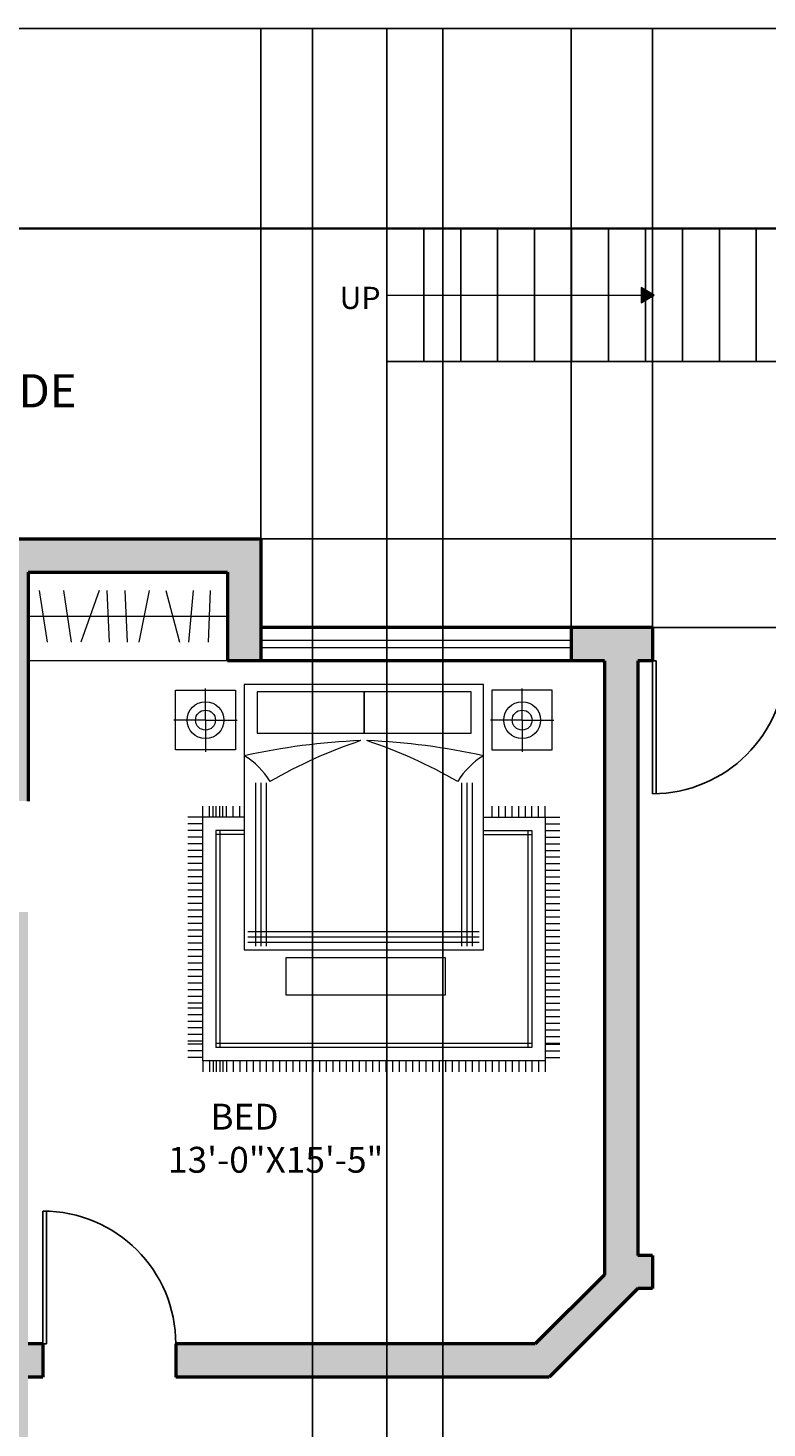
# Model space of a CAD drawing. Units: inches. Extents: x 2447 to 3157, y 2799 to 3988.
# Tile 8 of 9: x 2735 to 2935, y 3609 to 3988. Entities that reach past the tile are written whole.
import ezdxf

# ---------------------------------------------------------------- set-up
doc = ezdxf.new("R2010")
doc.units = ezdxf.units.IN
for name, color, linetype, lineweight in [('A-ANNO-DIMS', 2, 'Continuous', 18), ('A-ANNO-SYMB', 2, 'Continuous', 18), ('A-AREA-IDEN', 7, 'Continuous', 25), ('A-DOOR', 3, 'Continuous', 25), ('A-FLOR-CASE', 8, 'Continuous', 20), ('A-FLOR-STRS', 7, 'Continuous', 25), ('A-FURN', 8, 'Continuous', 18), ('A-GLAZ', 4, 'Continuous', 18), ('A-WALL', 7, 'Continuous', 50), ('A-WALL-PATT', 252, 'Continuous', 13), ('C-PROP', 6, 'Continuous', 35)]:
    doc.layers.add(name, color=color, linetype=linetype, lineweight=lineweight)
doc.styles.get("Standard").update_dxf_attribs({"font": 'arial.ttf'})
doc.dimstyles.get("Standard").update_dxf_attribs({"dimtxt": 0.18, "dimasz": 0.18, "dimexe": 0.18, "dimexo": 0.0625, "dimgap": 0.09, "dimtad": 0, "dimtih": 1, "dimtoh": 1, "dimdec": 4, "dimzin": 0, "dimdsep": 46, "dimtxsty": 'Standard', "dimcen": 0.09, "dimadec": 0, "dimazin": 0, "dimtfac": 1, "dimtdec": 4, "dimtofl": 0, "dimtmove": 0, "dimatfit": 3, "dimfxl": 1, "dimtolj": 1, "dimtzin": 0, "dimarcsym": 0})

# ---------------------------------------------------------------- blocks, each defined once
blk = doc.blocks.new('A$C462B680F')
for p, q in [((0.011, 2.874, -0.291), (0.465, 2.874, -0.291)), ((0.011, 2.424, -0.291), (0.011, 2.874, -0.291)), ((0.238, 2.649, -0.561), (0.238, 2.887, -0.561)), ((0.465, 2.874, -0.291), (0.465, 2.424, -0.291)), ((2.33, 2.918, -0.291), (0.53, 2.918, -0.291)), ((0.53, 2.918, -0.291), (0.53, 0.918, -0.291)), ((1.434, 2.861, -0.291), (0.627, 2.861, -0.291)), ((0.627, 2.861, -0.291), (0.627, 2.55, -0.291)), ((1.43, 2.861, -0.291), (1.43, 2.55, -0.291)), ((2.237, 2.861, -0.291), (1.43, 2.861, -0.291)), ((1.434, 2.55, -0.291), (1.434, 2.861, -0.291)), ((2.237, 2.55, -0.291), (2.237, 2.861, -0.291)), ((2.33, 0.918, -0.291), (2.33, 2.918, -0.291)), ((2.849, 2.874, -0.291), (2.395, 2.874, -0.291)), ((2.395, 2.874, -0.291), (2.395, 2.424, -0.291)), ((2.622, 2.649, -0.561), (2.622, 2.887, -0.561)), ((2.849, 2.424, -0.291), (2.849, 2.874, -0.291)), ((0.238, 2.649, -0.561), (0, 2.649, -0.561)), ((0.238, 2.649, -0.561), (0.238, 2.411, -0.561)), ((0.238, 2.649, -0.561), (0.476, 2.649, -0.561)), ((2.622, 2.649, -0.561), (2.384, 2.649, -0.561)), ((2.622, 2.649, -0.561), (2.622, 2.411, -0.561)), ((2.622, 2.649, -0.561), (2.861, 2.649, -0.561)), ((0.627, 2.55, -0.291), (1.434, 2.55, -0.291)), ((1.43, 2.55, -0.291), (2.237, 2.55, -0.291)), ((0.465, 2.424, -0.291), (0.011, 2.424, -0.291)), ((2.395, 2.424, -0.291), (2.849, 2.424, -0.291)), ((0.615, 2.176, -0.291), (0.615, 0.947, -0.291)), ((0.655, 2.176, -0.291), (0.655, 0.947, -0.291)), ((0.695, 2.176, -0.291), (0.695, 0.947, -0.291)), ((2.165, 2.176, -0.291), (2.165, 0.947, -0.291)), ((2.205, 2.176, -0.291), (2.205, 0.947, -0.291)), ((2.245, 2.176, -0.291), (2.245, 0.947, -0.291)), ((0.215, 1.918, -0.291), (0.105, 1.918, -0.291)), ((0.215, 1.918, -0.291), (0.215, 0.082, -0.291)), ((0.53, 1.918, -0.291), (0.215, 1.918, -0.291)), ((0.219, 1.918, -0.291), (0.219, 2, -0.291)), ((0.269, 1.918, -0.291), (0.269, 2, -0.291)), ((0.296, 1.918, -0.291), (0.296, 2, -0.291)), ((0.319, 1.918, -0.291), (0.319, 2, -0.291)), ((0.346, 1.918, -0.291), (0.346, 2, -0.291)), ((0.369, 1.918, -0.291), (0.369, 2, -0.291)), ((0.396, 1.918, -0.291), (0.396, 2, -0.291)), ((0.446, 1.918, -0.291), (0.446, 2, -0.291)), ((0.496, 1.918, -0.291), (0.496, 2, -0.291)), ((2.33, 1.918, -0.291), (2.796, 1.918, -0.291)), ((2.396, 1.918, -0.291), (2.396, 2, -0.291)), ((2.446, 1.918, -0.291), (2.446, 2, -0.291)), ((2.496, 1.918, -0.291), (2.496, 2, -0.291)), ((2.546, 1.918, -0.291), (2.546, 2, -0.291)), ((2.596, 1.918, -0.291), (2.596, 2, -0.291)), ((2.646, 1.918, -0.291), (2.646, 2, -0.291)), ((2.696, 1.918, -0.291), (2.696, 2, -0.291)), ((2.746, 1.918, -0.291), (2.746, 2, -0.291)), ((2.796, 1.918, -0.291), (2.796, 2, -0.291)), ((2.796, 1.918, -0.291), (2.796, 0.082, -0.291)), ((2.796, 1.918, -0.291), (2.906, 1.918, -0.291)), ((0.215, 1.868, -0.291), (0.105, 1.868, -0.291)), ((0.215, 1.818, -0.291), (0.105, 1.818, -0.291)), ((0.315, 1.818, -0.291), (0.315, 0.182, -0.291)), ((0.53, 1.818, -0.291), (0.315, 1.818, -0.291)), ((0.345, 1.818, -0.291), (0.345, 0.182, -0.291)), ((2.33, 1.818, -0.291), (2.696, 1.818, -0.291)), ((2.666, 1.818, -0.291), (2.666, 0.182, -0.291)), ((2.696, 1.818, -0.291), (2.696, 0.182, -0.291)), ((2.796, 1.868, -0.291), (2.906, 1.868, -0.291)), ((2.796, 1.818, -0.291), (2.906, 1.818, -0.291)), ((0.215, 1.768, -0.291), (0.105, 1.768, -0.291)), ((0.215, 1.718, -0.291), (0.105, 1.718, -0.291)), ((0.53, 1.788, -0.291), (0.315, 1.788, -0.291)), ((2.33, 1.788, -0.291), (2.696, 1.788, -0.291)), ((2.796, 1.768, -0.291), (2.906, 1.768, -0.291)), ((2.796, 1.718, -0.291), (2.906, 1.718, -0.291)), ((0.215, 1.668, -0.291), (0.105, 1.668, -0.291)), ((0.215, 1.618, -0.291), (0.105, 1.618, -0.291)), ((2.796, 1.668, -0.291), (2.906, 1.668, -0.291)), ((2.796, 1.618, -0.291), (2.906, 1.618, -0.291)), ((0.215, 1.568, -0.291), (0.105, 1.568, -0.291)), ((0.215, 1.518, -0.291), (0.105, 1.518, -0.291)), ((2.796, 1.568, -0.291), (2.906, 1.568, -0.291)), ((2.796, 1.518, -0.291), (2.906, 1.518, -0.291)), ((0.215, 1.468, -0.291), (0.105, 1.468, -0.291)), ((0.215, 1.418, -0.291), (0.105, 1.418, -0.291)), ((2.796, 1.468, -0.291), (2.906, 1.468, -0.291)), ((2.796, 1.418, -0.291), (2.906, 1.418, -0.291)), ((0.215, 1.368, -0.291), (0.105, 1.368, -0.291)), ((0.215, 1.318, -0.291), (0.105, 1.318, -0.291)), ((0.215, 1.268, -0.291), (0.105, 1.268, -0.291)), ((2.796, 1.368, -0.291), (2.906, 1.368, -0.291)), ((2.796, 1.318, -0.291), (2.906, 1.318, -0.291)), ((2.796, 1.268, -0.291), (2.906, 1.268, -0.291)), ((0.215, 1.218, -0.291), (0.105, 1.218, -0.291)), ((0.215, 1.168, -0.291), (0.105, 1.168, -0.291)), ((2.796, 1.218, -0.291), (2.906, 1.218, -0.291)), ((2.796, 1.168, -0.291), (2.906, 1.168, -0.291)), ((0.215, 1.118, -0.291), (0.105, 1.118, -0.291)), ((0.215, 1.068, -0.291), (0.105, 1.068, -0.291)), ((0.558, 1.057, -0.291), (2.299, 1.057, -0.291)), ((2.796, 1.118, -0.291), (2.906, 1.118, -0.291)), ((2.796, 1.068, -0.291), (2.906, 1.068, -0.291)), ((0.215, 1.018, -0.291), (0.105, 1.018, -0.291)), ((0.215, 0.968, -0.291), (0.105, 0.968, -0.291)), ((0.558, 1.017, -0.291), (2.299, 1.017, -0.291)), ((0.558, 0.977, -0.291), (2.299, 0.977, -0.291)), ((2.796, 1.018, -0.291), (2.906, 1.018, -0.291)), ((2.796, 0.968, -0.291), (2.906, 0.968, -0.291)), ((0.215, 0.918, -0.291), (0.105, 0.918, -0.291)), ((0.215, 0.868, -0.291), (0.105, 0.868, -0.291)), ((0.53, 0.918, -0.291), (2.33, 0.918, -0.291)), ((0.844, 0.859, -0.291), (0.844, 0.579, -0.291)), ((2.044, 0.859, -0.291), (0.844, 0.859, -0.291)), ((2.044, 0.579, -0.291), (2.044, 0.859, -0.291)), ((2.796, 0.918, -0.291), (2.906, 0.918, -0.291)), ((2.796, 0.868, -0.291), (2.906, 0.868, -0.291)), ((0.215, 0.818, -0.291), (0.105, 0.818, -0.291)), ((0.215, 0.768, -0.291), (0.105, 0.768, -0.291)), ((2.796, 0.818, -0.291), (2.906, 0.818, -0.291)), ((2.796, 0.768, -0.291), (2.906, 0.768, -0.291)), ((0.215, 0.718, -0.291), (0.105, 0.718, -0.291)), ((0.215, 0.668, -0.291), (0.105, 0.668, -0.291)), ((2.796, 0.718, -0.291), (2.906, 0.718, -0.291)), ((2.796, 0.668, -0.291), (2.906, 0.668, -0.291)), ((0.215, 0.618, -0.291), (0.105, 0.618, -0.291)), ((0.215, 0.568, -0.291), (0.105, 0.568, -0.291)), ((0.844, 0.579, -0.291), (2.044, 0.579, -0.291)), ((2.796, 0.618, -0.291), (2.906, 0.618, -0.291)), ((2.796, 0.568, -0.291), (2.906, 0.568, -0.291)), ((0.215, 0.518, -0.291), (0.105, 0.518, -0.291)), ((0.215, 0.48, -0.291), (0.105, 0.48, -0.291)), ((0.215, 0.43, -0.291), (0.105, 0.43, -0.291)), ((2.796, 0.518, -0.291), (2.906, 0.518, -0.291)), ((2.796, 0.516, -0.291), (2.906, 0.516, -0.291)), ((2.796, 0.466, -0.291), (2.906, 0.466, -0.291)), ((0.215, 0.38, -0.291), (0.105, 0.38, -0.291)), ((0.215, 0.33, -0.291), (0.105, 0.33, -0.291)), ((2.796, 0.416, -0.291), (2.906, 0.416, -0.291)), ((2.796, 0.366, -0.291), (2.906, 0.366, -0.291)), ((0.215, 0.28, -0.291), (0.105, 0.28, -0.291)), ((0.215, 0.23, -0.291), (0.105, 0.23, -0.291)), ((2.696, 0.212, -0.291), (0.315, 0.212, -0.291)), ((2.796, 0.316, -0.291), (2.906, 0.316, -0.291)), ((2.796, 0.266, -0.291), (2.906, 0.266, -0.291)), ((2.796, 0.216, -0.291), (2.906, 0.216, -0.291)), ((0.215, 0.207, -0.291), (0.105, 0.207, -0.291)), ((0.215, 0.207, -0.291), (0.105, 0.207, -0.291)), ((0.215, 0.157, -0.291), (0.105, 0.157, -0.291)), ((0.215, 0.107, -0.291), (0.105, 0.107, -0.291)), ((2.696, 0.182, -0.291), (0.315, 0.182, -0.291)), ((2.796, 0.207, -0.291), (2.906, 0.207, -0.291)), ((2.796, 0.207, -0.291), (2.906, 0.207, -0.291)), ((2.796, 0.157, -0.291), (2.906, 0.157, -0.291)), ((2.796, 0.107, -0.291), (2.906, 0.107, -0.291)), ((2.796, 0.082, -0.291), (0.215, 0.082, -0.291)), ((0.219, 0.082, -0.291), (0.219, 0, -0.291)), ((0.269, 0.082, -0.291), (0.269, 0, -0.291)), ((0.296, 0.082, -0.291), (0.296, 0, -0.291)), ((0.319, 0.082, -0.291), (0.319, 0, -0.291)), ((0.346, 0.082, -0.291), (0.346, 0, -0.291)), ((0.369, 0.082, -0.291), (0.369, 0, -0.291)), ((0.396, 0.082, -0.291), (0.396, 0, -0.291)), ((0.446, 0.082, -0.291), (0.446, 0, -0.291)), ((0.496, 0.082, -0.291), (0.496, 0, -0.291)), ((0.546, 0.082, -0.291), (0.546, 0, -0.291)), ((0.596, 0.082, -0.291), (0.596, 0, -0.291)), ((0.646, 0.082, -0.291), (0.646, 0, -0.291)), ((0.696, 0.082, -0.291), (0.696, 0, -0.291)), ((0.746, 0.082, -0.291), (0.746, 0, -0.291)), ((0.796, 0.082, -0.291), (0.796, 0, -0.291)), ((0.846, 0.082, -0.291), (0.846, 0, -0.291)), ((0.896, 0.082, -0.291), (0.896, 0, -0.291)), ((0.946, 0.082, -0.291), (0.946, 0, -0.291)), ((0.996, 0.082, -0.291), (0.996, 0, -0.291)), ((1.046, 0.082, -0.291), (1.046, 0, -0.291)), ((1.096, 0.082, -0.291), (1.096, 0, -0.291)), ((1.146, 0.082, -0.291), (1.146, 0, -0.291)), ((1.196, 0.082, -0.291), (1.196, 0, -0.291)), ((1.246, 0.082, -0.291), (1.246, 0, -0.291)), ((1.296, 0.082, -0.291), (1.296, 0, -0.291)), ((1.346, 0.082, -0.291), (1.346, 0, -0.291)), ((1.346, 0.082, -0.291), (1.346, 0, -0.291)), ((1.396, 0.082, -0.291), (1.396, 0, -0.291)), ((1.396, 0.082, -0.291), (1.396, 0, -0.291)), ((1.446, 0.082, -0.291), (1.446, 0, -0.291)), ((1.446, 0.082, -0.291), (1.446, 0, -0.291)), ((1.496, 0.082, -0.291), (1.496, 0, -0.291)), ((1.496, 0.082, -0.291), (1.496, 0, -0.291)), ((1.546, 0.082, -0.291), (1.546, 0, -0.291)), ((1.596, 0.082, -0.291), (1.596, 0, -0.291)), ((1.646, 0.082, -0.291), (1.646, 0, -0.291)), ((1.696, 0.082, -0.291), (1.696, 0, -0.291)), ((1.746, 0.082, -0.291), (1.746, 0, -0.291)), ((1.796, 0.082, -0.291), (1.796, 0, -0.291)), ((1.846, 0.082, -0.291), (1.846, 0, -0.291)), ((1.846, 0.082, -0.291), (1.846, 0, -0.291)), ((1.896, 0.082, -0.291), (1.896, 0, -0.291)), ((1.946, 0.082, -0.291), (1.946, 0, -0.291)), ((1.996, 0.082, -0.291), (1.996, 0, -0.291)), ((2.046, 0.082, -0.291), (2.046, 0, -0.291)), ((2.096, 0.082, -0.291), (2.096, 0, -0.291)), ((2.146, 0.082, -0.291), (2.146, 0, -0.291)), ((2.196, 0.082, -0.291), (2.196, 0, -0.291)), ((2.246, 0.082, -0.291), (2.246, 0, -0.291)), ((2.296, 0.082, -0.291), (2.296, 0, -0.291)), ((2.346, 0.082, -0.291), (2.346, 0, -0.291)), ((2.396, 0.082, -0.291), (2.396, 0, -0.291)), ((2.446, 0.082, -0.291), (2.446, 0, -0.291)), ((2.496, 0.082, -0.291), (2.496, 0, -0.291)), ((2.546, 0.082, -0.291), (2.546, 0, -0.291)), ((2.596, 0.082, -0.291), (2.596, 0, -0.291)), ((2.646, 0.082, -0.291), (2.646, 0, -0.291)), ((2.696, 0.082, -0.291), (2.696, 0, -0.291)), ((2.746, 0.082, -0.291), (2.746, 0, -0.291)), ((2.796, 0.082, -0.291), (2.796, 0, -0.291))]:
    blk.add_line(p, q)
for centre, radius in [((0.238, 2.649, -0.561), 0.139), ((2.622, 2.649, -0.561), 0.139), ((0.238, 2.649, -0.561), 0.075), ((2.622, 2.649, -0.561), 0.075)]:
    blk.add_circle(centre, radius)
for centre, radius, start, end in [((1.618, -2.572, -0.291), 5.071, 92.3872, 102.3913), ((2.601, -1.074, -0.291), 3.763, 108.5127, 119.9306), ((1.243, -2.572, -0.291), 5.071, 77.6087, 87.6128), ((0.259, -1.074, -0.291), 3.763, 60.0694, 71.4873), ((0.231, 1.886, -0.291), 0.578, 31.4118, 58.8491), ((2.63, 1.886, -0.291), 0.578, 121.1509, 148.5882)]:
    blk.add_arc(centre, radius, start, end)
blk = doc.blocks.new('DOOR-SWING-36IN')
for p, q in [((0, 0), (0, 36)), ((1, 0), (1, 35.99)), ((1, 0), (0, 0))]:
    blk.add_line(p, q)
blk.add_arc((0, 0), 36, 0, 90)
blk = doc.blocks.new('*D46')
at = {"layer": 'A-ANNO-DIMS', "color": 0, "lineweight": -2, "transparency": 16777216}
for p, q in [((2561.37, 3849.76), (2561.37, 3988.03)), ((3046.37, 3825.76), (3046.37, 3988.03)), ((2561.55, 3987.85), (2803.57, 3987.85)), ((3046.19, 3987.85), (2804.16, 3987.85))]:
    blk.add_line(p, q, dxfattribs=at)
at = {"layer": 'A-ANNO-DIMS', "color": 0, "transparency": 16777216}
for points in [[(2561.55, 3987.88), (2561.55, 3987.82), (2561.37, 3987.85)], [(3046.19, 3987.88), (3046.19, 3987.82), (3046.37, 3987.85)]]:
    blk.add_solid(points, dxfattribs=at)
at = {"layer": 'Defpoints', "color": 0, "transparency": 16777216}
for p in [(3046.37, 3987.85), (2561.37, 3849.7), (3046.37, 3825.7)]:
    blk.add_point(p, dxfattribs=at)
at = {"layer": 'A-ANNO-DIMS', "color": 0, "transparency": 16777216, "insert": (2803.87, 3987.85), "char_height": 0.18, "attachment_point": 5}
blk.add_mtext('\\A1;485', dxfattribs=at)
blk = doc.blocks.new('*D47')
at = {"layer": 'A-ANNO-DIMS', "color": 0, "lineweight": -2, "transparency": 16777216}
for p, q in [((2798.43, 3849.7), (3156.7, 3849.7)), ((3156.52, 3849.52), (3156.52, 3487.38)), ((3156.52, 3124.88), (3156.52, 3487.02)), ((3046.43, 3124.7), (3156.7, 3124.7))]:
    blk.add_line(p, q, dxfattribs=at)
at = {"layer": 'A-ANNO-DIMS', "color": 0, "transparency": 16777216}
for points in [[(3156.49, 3849.52), (3156.55, 3849.52), (3156.52, 3849.7)], [(3156.49, 3124.88), (3156.55, 3124.88), (3156.52, 3124.7)]]:
    blk.add_solid(points, dxfattribs=at)
at = {"layer": 'Defpoints', "color": 0, "transparency": 16777216}
for p in [(2798.37, 3849.7), (3156.52, 3849.7), (3046.37, 3124.7)]:
    blk.add_point(p, dxfattribs=at)
at = {"layer": 'A-ANNO-DIMS', "color": 0, "transparency": 16777216, "insert": (3156.52, 3487.2), "char_height": 0.18, "attachment_point": 5}
blk.add_mtext('\\A1;725', dxfattribs=at)
blk = doc.blocks.new('*D50')
at = {"layer": 'A-ANNO-DIMS', "color": 0, "lineweight": -2, "transparency": 16777216}
for p, q in [((2832.46, 3897.64), (2832.46, 2799.37)), ((2942.46, 3897.64), (2942.46, 2799.37)), ((2832.64, 2799.55), (2887.18, 2799.55)), ((2942.28, 2799.55), (2887.74, 2799.55))]:
    blk.add_line(p, q, dxfattribs=at)
at = {"layer": 'A-ANNO-DIMS', "color": 0, "transparency": 16777216}
for points in [[(2832.64, 2799.58), (2832.64, 2799.52), (2832.46, 2799.55)], [(2942.28, 2799.58), (2942.28, 2799.52), (2942.46, 2799.55)]]:
    blk.add_solid(points, dxfattribs=at)
at = {"layer": 'Defpoints', "color": 0, "transparency": 16777216}
for p in [(2832.46, 3897.7), (2942.46, 3897.7), (2942.46, 2799.55)]:
    blk.add_point(p, dxfattribs=at)
at = {"layer": 'A-ANNO-DIMS', "color": 0, "transparency": 16777216, "insert": (2887.46, 2799.55), "char_height": 0.18, "attachment_point": 5}
blk.add_mtext('\\A1;110', dxfattribs=at)
blk = doc.blocks.new('*D52')
at = {"layer": 'A-ANNO-DIMS', "color": 0, "lineweight": -2, "transparency": 16777216}
for p, q in [((2501.37, 3933.76), (2501.37, 3988.03)), ((2832.46, 3933.76), (2832.46, 3988.03)), ((2501.55, 3987.85), (2666.54, 3987.85)), ((2832.28, 3987.85), (2667.29, 3987.85))]:
    blk.add_line(p, q, dxfattribs=at)
at = {"layer": 'A-ANNO-DIMS', "color": 0, "transparency": 16777216}
for points in [[(2501.55, 3987.88), (2501.55, 3987.82), (2501.37, 3987.85)], [(2832.28, 3987.88), (2832.28, 3987.82), (2832.46, 3987.85)]]:
    blk.add_solid(points, dxfattribs=at)
at = {"layer": 'Defpoints', "color": 0, "transparency": 16777216}
for p in [(2832.46, 3987.85), (2501.37, 3933.7), (2832.46, 3933.7)]:
    blk.add_point(p, dxfattribs=at)
at = {"layer": 'A-ANNO-DIMS', "color": 0, "transparency": 16777216, "insert": (2666.91, 3987.85), "char_height": 0.18, "attachment_point": 5}
blk.add_mtext('\\A1;331.1', dxfattribs=at)
blk = doc.blocks.new('*D62')
at = {"layer": 'A-ANNO-DIMS', "color": 0, "lineweight": -2, "transparency": 16777216}
for p, q in [((2798.43, 3849.7), (3156.7, 3849.7)), ((3156.52, 3849.52), (3156.52, 3837.88)), ((3156.52, 3825.88), (3156.52, 3837.52)), ((2798.43, 3825.7), (3156.7, 3825.7))]:
    blk.add_line(p, q, dxfattribs=at)
at = {"layer": 'A-ANNO-DIMS', "color": 0, "transparency": 16777216}
for points in [[(3156.49, 3849.52), (3156.55, 3849.52), (3156.52, 3849.7)], [(3156.49, 3825.88), (3156.55, 3825.88), (3156.52, 3825.7)]]:
    blk.add_solid(points, dxfattribs=at)
at = {"layer": 'Defpoints', "color": 0, "transparency": 16777216}
for p in [(2798.37, 3849.7), (2798.37, 3825.7), (3156.52, 3825.7)]:
    blk.add_point(p, dxfattribs=at)
at = {"layer": 'A-ANNO-DIMS', "color": 0, "transparency": 16777216, "insert": (3156.52, 3837.7), "char_height": 0.18, "attachment_point": 5}
blk.add_mtext('\\A1;24', dxfattribs=at)
blk = doc.blocks.new('*D63')
at = {"layer": 'A-ANNO-DIMS', "color": 0, "lineweight": -2, "transparency": 16777216}
for p, q in [((2798.37, 3825.76), (2798.37, 3988.03)), ((2882.37, 3825.76), (2882.37, 3988.03)), ((2798.55, 3987.85), (2840.15, 3987.85)), ((2882.19, 3987.85), (2840.59, 3987.85))]:
    blk.add_line(p, q, dxfattribs=at)
at = {"layer": 'A-ANNO-DIMS', "color": 0, "transparency": 16777216}
for points in [[(2798.55, 3987.88), (2798.55, 3987.82), (2798.37, 3987.85)], [(2882.19, 3987.88), (2882.19, 3987.82), (2882.37, 3987.85)]]:
    blk.add_solid(points, dxfattribs=at)
at = {"layer": 'Defpoints', "color": 0, "transparency": 16777216}
for p in [(2882.37, 3987.85), (2798.37, 3825.7), (2882.37, 3825.7)]:
    blk.add_point(p, dxfattribs=at)
at = {"layer": 'A-ANNO-DIMS', "color": 0, "transparency": 16777216, "insert": (2840.37, 3987.85), "char_height": 0.18, "attachment_point": 5}
blk.add_mtext('\\A1;84', dxfattribs=at)
blk = doc.blocks.new('*D64')
at = {"layer": 'A-ANNO-DIMS', "color": 0, "lineweight": -2, "transparency": 16777216}
for p, q in [((2882.37, 3825.76), (2882.37, 3988.03)), ((2904.37, 3825.76), (2904.37, 3988.03)), ((2882.55, 3987.85), (2893.15, 3987.85)), ((2904.19, 3987.85), (2893.59, 3987.85))]:
    blk.add_line(p, q, dxfattribs=at)
at = {"layer": 'A-ANNO-DIMS', "color": 0, "transparency": 16777216}
for points in [[(2882.55, 3987.88), (2882.55, 3987.82), (2882.37, 3987.85)], [(2904.19, 3987.88), (2904.19, 3987.82), (2904.37, 3987.85)]]:
    blk.add_solid(points, dxfattribs=at)
at = {"layer": 'Defpoints', "color": 0, "transparency": 16777216}
for p in [(2904.37, 3987.85), (2882.37, 3825.7), (2904.37, 3825.7)]:
    blk.add_point(p, dxfattribs=at)
at = {"layer": 'A-ANNO-DIMS', "color": 0, "transparency": 16777216, "insert": (2893.37, 3987.85), "char_height": 0.18, "attachment_point": 5}
blk.add_mtext('\\A1;22', dxfattribs=at)
blk = doc.blocks.new('*D73')
at = {"layer": 'A-ANNO-DIMS', "color": 0, "lineweight": -2, "transparency": 16777216}
for p, q in [((2812.37, 3160.03), (2812.37, 3988.03)), ((2847.64, 3124.76), (2847.64, 3988.03)), ((2812.55, 3987.85), (2829.61, 3987.85)), ((2847.46, 3987.85), (2830.4, 3987.85))]:
    blk.add_line(p, q, dxfattribs=at)
at = {"layer": 'A-ANNO-DIMS', "color": 0, "transparency": 16777216}
for points in [[(2812.55, 3987.88), (2812.55, 3987.82), (2812.37, 3987.85)], [(2847.46, 3987.88), (2847.46, 3987.82), (2847.64, 3987.85)]]:
    blk.add_solid(points, dxfattribs=at)
at = {"layer": 'Defpoints', "color": 0, "transparency": 16777216}
for p in [(2847.64, 3987.85), (2812.37, 3159.97), (2847.64, 3124.7)]:
    blk.add_point(p, dxfattribs=at)
at = {"layer": 'A-ANNO-DIMS', "color": 0, "transparency": 16777216, "insert": (2830, 3987.85), "char_height": 0.18, "attachment_point": 5}
blk.add_mtext('\\A1;35.27', dxfattribs=at)
blk = doc.blocks.new('*D76')
at = {"layer": 'A-ANNO-DIMS', "color": 0, "lineweight": -2, "transparency": 16777216}
for p, q in [((2847.64, 3124.76), (2847.64, 3988.03)), ((2971.17, 3124.76), (2971.17, 3988.03)), ((2847.82, 3987.85), (2908.95, 3987.85)), ((2970.99, 3987.85), (2909.86, 3987.85))]:
    blk.add_line(p, q, dxfattribs=at)
at = {"layer": 'A-ANNO-DIMS', "color": 0, "transparency": 16777216}
for points in [[(2847.82, 3987.88), (2847.82, 3987.82), (2847.64, 3987.85)], [(2970.99, 3987.88), (2970.99, 3987.82), (2971.17, 3987.85)]]:
    blk.add_solid(points, dxfattribs=at)
at = {"layer": 'Defpoints', "color": 0, "transparency": 16777216}
for p in [(2971.17, 3987.85), (2847.64, 3124.7), (2971.17, 3124.7)]:
    blk.add_point(p, dxfattribs=at)
at = {"layer": 'A-ANNO-DIMS', "color": 0, "transparency": 16777216, "insert": (2909.4, 3987.85), "char_height": 0.18, "attachment_point": 5}
blk.add_mtext('\\A1;123.53', dxfattribs=at)

msp = doc.modelspace()

# ---------------------------------------------------------------- hatches: boundary and pattern name
at = {"layer": 'A-ANNO-SYMB'}
h = msp.add_hatch(color=256, dxfattribs=at)
h.dxf.hatch_style = 1
h.paths.add_polyline_path([(2904.8279, 3915.7002), (2901.27, 3917.7544), (2901.27, 3913.6461)])
at = {"layer": 'A-WALL-PATT'}
h = msp.add_hatch(color=256, dxfattribs=at)
h.dxf.hatch_style = 1
h.paths.add_polyline_path([(2570.3672, 3550.7002), (2726.3672, 3550.7002), (2726.3672, 3370.7002), (2722.3672, 3370.7002), (2722.3672, 3365.7002), (2739.3672, 3365.7002), (2739.3672, 3374.7002), (2735.3672, 3374.7002), (2735.3672, 3563.7002), (2726.3672, 3563.7002), (2726.3672, 3559.7002), (2570.3672, 3559.7002), (2570.3672, 3599.2479), (2561.3672, 3599.2479), (2561.3672, 3508.7002), (2570.3672, 3508.7002)])
h.paths.add_polyline_path([(2570.3672, 3412.7002), (2561.3672, 3412.7002), (2561.3672, 3331.9279), (2570.3672, 3331.9279), (2570.3672, 3365.7002), (2666.3672, 3365.7002), (2666.3672, 3361.7002), (2671.3672, 3361.7002), (2671.3672, 3365.7002), (2686.3672, 3365.7002), (2686.3672, 3370.7002), (2570.3672, 3370.7002)])
h.paths.add_polyline_path([(2965.3672, 3430.7002), (2961.3672, 3430.7002), (2961.3672, 3434.7002), (2952.3672, 3434.7002), (2952.3672, 3430.7002), (2847.6393, 3430.7002), (2812.3672, 3395.4282), (2812.3672, 3374.7002), (2781.3672, 3374.7002), (2781.3672, 3365.7002), (2812.3672, 3365.7002), (2812.3672, 3347.7002), (2821.3672, 3347.7002), (2821.3672, 3391.7002), (2851.3672, 3421.7002), (2965.3672, 3421.7002)])
h.paths.add_polyline_path([(3046.3672, 3430.7002), (3033.3672, 3430.7002), (3033.3672, 3421.7002), (3037.3672, 3421.7002), (3037.3672, 3133.7002), (2971.1661, 3133.7002), (2971.1661, 3124.7002), (3046.3672, 3124.7002)])
h.paths.add_polyline_path([(3046.3672, 3825.7002), (3005.5801, 3825.7002), (3005.5801, 3816.7002), (3037.3672, 3816.7002), (3037.3672, 3655.7002), (2940.3672, 3655.7002), (2940.3672, 3646.7002), (3037.3672, 3646.7002), (3037.3672, 3514.7002), (3033.3672, 3514.7002), (3033.3672, 3505.7002), (3046.3672, 3505.7002)])
h.paths.add_polyline_path([(2821.3672, 3258.7002), (2812.3672, 3258.7002), (2812.3672, 3240.7002), (2808.3672, 3240.7002), (2808.3672, 3231.7002), (2812.3672, 3231.7002), (2812.3672, 3223.0688), (2821.3672, 3223.0688)])
h.paths.add_polyline_path([(2766.3672, 3240.7002), (2707.3672, 3240.7002), (2707.3672, 3234.4466, -1), (2570.3672, 3234.4466), (2570.3672, 3240.5271), (2561.3672, 3240.5271), (2561.3672, 3234.4466, 0.98243292), (2716.3185, 3231.7002), (2766.3672, 3231.7002)])
h.paths.add_polyline_path([(2570.3672, 3307.9279), (2561.3672, 3307.9279), (2561.3672, 3281.7773), (2570.3672, 3281.7773), (2570.3672, 3284.7002), (2671.3672, 3284.7002), (2671.3672, 3331.7002), (2666.3672, 3331.7002), (2666.3672, 3293.7002), (2570.3672, 3293.7002)])
h.paths.add_polyline_path([(2570.3672, 3739.7002), (2574.3672, 3739.7002), (2574.3672, 3744.7002), (2570.3672, 3744.7002), (2570.3672, 3840.7002), (2614.3672, 3840.7002), (2614.3672, 3849.7002), (2561.3672, 3849.7002), (2561.3672, 3671.2479), (2570.3672, 3671.2479)])
h.paths.add_polyline_path([(2735.3672, 3840.7002), (2789.3672, 3840.7002), (2789.3672, 3816.7002), (2798.3672, 3816.7002), (2798.3672, 3849.7002), (2679.3672, 3849.7002), (2679.3672, 3840.7002), (2726.3672, 3840.7002), (2726.3672, 3778.7002), (2735.3672, 3778.7002)])
h.paths.add_polyline_path([(2651.3672, 3840.7002), (2655.3672, 3840.7002), (2655.3672, 3849.7002), (2638.3672, 3849.7002), (2638.3672, 3840.7002), (2642.3672, 3840.7002), (2642.3672, 3744.7002), (2610.3672, 3744.7002), (2610.3672, 3739.7002), (2726.3672, 3739.7002), (2726.3672, 3599.7002), (2735.3672, 3599.7002), (2735.3672, 3622.7002), (2739.3672, 3622.7002), (2739.3672, 3631.7002), (2735.3672, 3631.7002), (2735.3672, 3748.7002), (2726.3672, 3748.7002), (2726.3672, 3744.7002), (2651.3672, 3744.7002)])
h.paths.add_polyline_path([(2900.3672, 3816.7002), (2904.3672, 3816.7002), (2904.3672, 3825.7002), (2882.3672, 3825.7002), (2882.3672, 3816.7002), (2891.3672, 3816.7002), (2891.3672, 3650.4282), (2872.6393, 3631.7002), (2775.3672, 3631.7002), (2775.3672, 3622.7002), (2876.3672, 3622.7002), (2900.3672, 3646.7002), (2904.3672, 3646.7002), (2904.3672, 3655.7002), (2900.3672, 3655.7002)])
h.paths.add_polyline_path([(2957.5801, 3825.7002), (2940.3672, 3825.7002), (2940.3672, 3816.7002), (2957.5801, 3816.7002)], flags=17)

# ---------------------------------------------------------------- linework, layer by layer
at = {"layer": 'A-ANNO-SYMB'}
msp.add_line((2832.456, 3915.7002), (2901.27, 3915.7002), dxfattribs=at)
msp.add_lwpolyline([(2904.8279, 3915.7002), (2901.27, 3917.7544), (2901.27, 3913.6461)], close=True, dxfattribs=at)
at = {"layer": 'A-FLOR-CASE'}
for p, q in [((2738.3808, 3835.7002), (2740.5602, 3821.7002)), ((2745.0019, 3835.7002), (2747.0704, 3821.7002)), ((2754.6377, 3835.7002), (2749.6735, 3821.7002)), ((2756.6918, 3835.7002), (2757.3554, 3821.7002)), ((2761.5953, 3835.7002), (2762.1872, 3821.7002)), ((2768.1525, 3835.7002), (2765.3304, 3821.7002)), ((2772.6408, 3835.7002), (2776.37, 3821.7002)), ((2780.0998, 3835.7002), (2778.8262, 3821.7002)), ((2784.6877, 3835.7002), (2784.164, 3821.7002)), ((2789.3672, 3828.7002), (2735.3672, 3828.7002)), ((2789.3672, 3816.7002), (2735.3672, 3816.7002))]:
    msp.add_line(p, q, dxfattribs=at)
at = {"layer": 'A-FLOR-STRS'}
for p, q in [((2832.456, 3897.7002), (2832.456, 3933.7002)), ((2842.456, 3897.7002), (2842.456, 3933.7002)), ((2852.456, 3897.7002), (2852.456, 3933.7002)), ((2862.456, 3897.7002), (2862.456, 3933.7002)), ((2872.456, 3897.7002), (2872.456, 3933.7002)), ((2882.456, 3897.7002), (2882.456, 3933.7002)), ((2892.456, 3897.7002), (2892.456, 3933.7002)), ((2902.456, 3917.0696), (2902.456, 3933.7002)), ((2912.456, 3897.7002), (2912.456, 3933.7002)), ((2922.456, 3897.7002), (2922.456, 3933.7002)), ((2932.456, 3897.7002), (2932.456, 3933.7002)), ((2902.456, 3897.7002), (2902.456, 3914.3308)), ((2832.456, 3897.7002), (2942.456, 3897.7002))]:
    msp.add_line(p, q, dxfattribs=at)
at = {"layer": 'A-GLAZ'}
for p, q in [((2882.3672, 3822.2002), (2798.3672, 3822.2002)), ((2882.3672, 3820.2002), (2798.3672, 3820.2002))]:
    msp.add_line(p, q, dxfattribs=at)
at = {"layer": 'A-WALL'}
for p, q in [((2561.3672, 3849.7002), (2798.3672, 3849.7002)), ((2798.3672, 3849.7002), (2798.3672, 3816.7002)), ((2735.3672, 3840.7002), (2735.3672, 3778.7002)), ((2735.3672, 3840.7002), (2789.3672, 3840.7002)), ((2789.3672, 3840.7002), (2789.3672, 3816.7002)), ((2904.3672, 3825.7002), (2798.3672, 3825.7002)), ((2882.3672, 3825.7002), (2882.3672, 3816.7002)), ((2904.3672, 3825.7002), (2904.3672, 3816.7002)), ((2891.3672, 3816.7002), (2789.3672, 3816.7002)), ((2891.3672, 3816.7002), (2891.3672, 3650.4282)), ((2900.3672, 3816.7002), (2900.3672, 3655.7002)), ((2904.3672, 3816.7002), (2900.3672, 3816.7002)), ((2904.3672, 3655.7002), (2900.3672, 3655.7002)), ((2904.3672, 3655.7002), (2904.3672, 3646.7002)), ((2891.3672, 3650.4282), (2872.6393, 3631.7002)), ((2900.3672, 3646.7002), (2876.3672, 3622.7002)), ((2904.3672, 3646.7002), (2900.3672, 3646.7002)), ((2739.3672, 3631.7002), (2735.3672, 3631.7002)), ((2739.3672, 3631.7002), (2739.3672, 3622.7002)), ((2872.6393, 3631.7002), (2775.3672, 3631.7002)), ((2775.3672, 3631.7002), (2775.3672, 3622.7002)), ((2739.3672, 3622.7002), (2735.3672, 3622.7002)), ((2876.3672, 3622.7002), (2775.3672, 3622.7002))]:
    msp.add_line(p, q, dxfattribs=at)
at = {"layer": 'C-PROP'}
msp.add_line((2501.3672, 3933.7002), (3102.3672, 3933.7002), dxfattribs=at)

# ---------------------------------------------------------------- block references
at = {"layer": 'A-DOOR', "extrusion": (0, 0, -1), "zscale": -1, "rotation": 180}
msp.add_blockref('DOOR-SWING-36IN', (-2904.3672, 3816.7002), dxfattribs=at)
at = {"layer": 'A-DOOR'}
msp.add_blockref('DOOR-SWING-36IN', (2739.3672, 3631.7002), dxfattribs=at)
at = {"layer": 'A-FURN', "xscale": 35.94635118840503, "yscale": 35.94635118840503, "zscale": 35.94635118840503}
msp.add_blockref('A$C462B680F', (2774.8414, 3705.4043), dxfattribs=at)

# ---------------------------------------------------------------- texts
at = {"layer": 'A-ANNO-SYMB', "insert": (2819.6855, 3917.9542), "char_height": 6, "attachment_point": 1}
msp.add_mtext_dynamic_manual_height_columns('UP', width=27.277438, gutter_width=12.5, heights=[0], dxfattribs=at)
at = {"layer": 'A-AREA-IDEN', "attachment_point": 1}
for s, width, insert, char_height in [('PASSAGE 7\'-0" WIDE', 130.290701, (2632.7819, 3894.2968), 9), ('               {\\H2.8x;BED\\P13\'-0"X15\'-5"}', 87.127135, (2773.2588, 3696.7509), 2.5)]:
    msp.add_mtext_dynamic_manual_height_columns(s, width=width, gutter_width=12.5, heights=[0], dxfattribs=dict(at, insert=insert, char_height=char_height))

# ---------------------------------------------------------------- dimensions: what is measured, and where the dimension line sits
at = {"layer": 'A-ANNO-DIMS'}
for base, p1, p2, override, picture, middle in [((2832.456, 3987.8502), (2501.3672, 3933.7002), (2832.456, 3933.7002), {"dimdec": 1, "dimlfac": 1, "dimrnd": 0, "dimzin": 0, "dimdsep": 46, "dimlunit": 2}, '*D52', (2666.9116, 3987.8502)), ((3046.3672, 3987.8502), (2561.3672, 3849.7002), (3046.3672, 3825.7002), {"dimdec": 0, "dimlfac": 1, "dimrnd": 0, "dimzin": 0, "dimdsep": 46, "dimlunit": 2}, '*D46', (2803.8672, 3987.8502)), ((2882.3672, 3987.8502), (2798.3672, 3825.7002), (2882.3672, 3825.7002), {"dimdec": 0, "dimlfac": 1, "dimrnd": 0, "dimzin": 0, "dimdsep": 46, "dimlunit": 2}, '*D63', (2840.3672, 3987.8502)), ((2847.6393, 3987.8502), (2812.3672, 3159.9723), (2847.6393, 3124.7002), {"dimdec": 2, "dimlfac": 1, "dimrnd": 0, "dimzin": 0, "dimdsep": 46, "dimlunit": 2}, '*D73', (2830.0033, 3987.8502)), ((2971.1661, 3987.8502), (2847.6393, 3124.7002), (2971.1661, 3124.7002), {"dimdec": 2, "dimlfac": 1, "dimrnd": 0, "dimzin": 0, "dimdsep": 46, "dimlunit": 2}, '*D76', (2909.4027, 3987.8502)), ((2904.3672, 3987.8502), (2882.3672, 3825.7002), (2904.3672, 3825.7002), {"dimdec": 0, "dimlfac": 1, "dimrnd": 0, "dimzin": 0, "dimdsep": 46, "dimlunit": 2}, '*D64', (2893.3672, 3987.8502)), ((2942.456, 2799.5502), (2832.456, 3897.7002), (2942.456, 3897.7002), {"dimdec": 0, "dimlfac": 1, "dimrnd": 0, "dimzin": 0, "dimdsep": 46, "dimlunit": 2}, '*D50', (2887.456, 2799.5502))]:
    dim = msp.add_linear_dim(base=base, p1=p1, p2=p2, dimstyle='Standard', override=override, dxfattribs=at)
    dim.commit()
    dim.dimension.update_dxf_attribs({"geometry": picture, "text_midpoint": middle})
for base, p1, p2, picture, middle in [((3156.5172, 3849.7002), (3046.3672, 3124.7002), (2798.3672, 3849.7002), '*D47', (3156.5172, 3487.2002)), ((3156.5172, 3825.7002), (2798.3672, 3849.7002), (2798.3672, 3825.7002), '*D62', (3156.5172, 3837.7002))]:
    dim = msp.add_linear_dim(base=base, p1=p1, p2=p2, angle=90, dimstyle='Standard', override={"dimdec": 0, "dimlfac": 1, "dimrnd": 0, "dimzin": 0, "dimdsep": 46, "dimlunit": 2}, dxfattribs=at)
    dim.commit()
    dim.dimension.update_dxf_attribs({"geometry": picture, "text_midpoint": middle})

doc.saveas('drawing.dxf')
